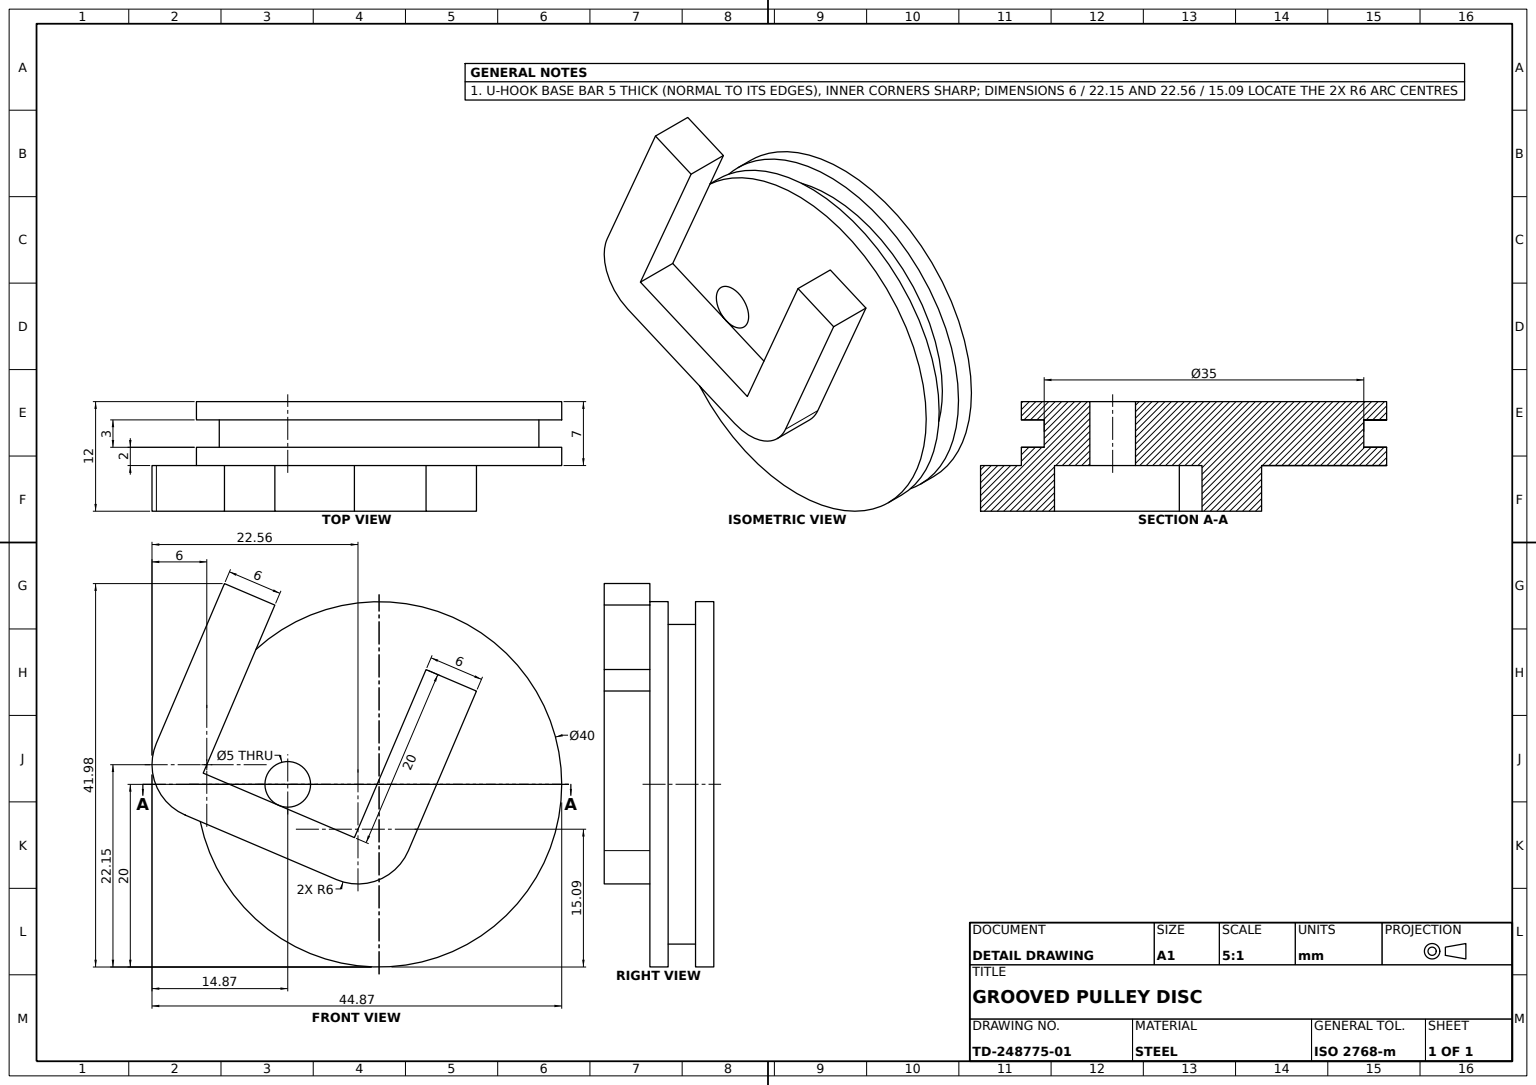
from build123d import *

# Parameters (mm, degrees)
DISC_PROFILE_40_R      = 20
DISC_40X7_DEPTH        = 3.5
RIM_GROOVE_PROFILE_W   = 3
RIM_GROOVE_PROFILE_H   = 2.5
THROUGH_HOLE_PROFILE_R = 2.5
THROUGH_HOLE_DEPTH     = 47
U_HOOK_BOSS_DEPTH      = 5


with BuildPart() as part:
    # Disc Profile Ø40 → Disc Ø40x7 (new, symmetric)
    with BuildSketch(Plane.XY):
        Circle(DISC_PROFILE_40_R)
    extrude(amount=DISC_40X7_DEPTH, both=True)

    # Rim Groove Profile → Rim Groove (revolve, cut)
    with BuildSketch(Plane(origin=(0, 0, 0), x_dir=(0, 0, -1), z_dir=(1, 0, 0)), mode=Mode.PRIVATE) as rim_groove_sk:
        with Locations((0, 18.75)):
            Rectangle(RIM_GROOVE_PROFILE_W, RIM_GROOVE_PROFILE_H)
    revolve(rim_groove_sk.sketch.rotate(Axis((0, 0, 14.756637323), (0, 0, -1)), 90), axis=Axis((0, 0, 14.756637323), (0, 0, -1)), mode=Mode.SUBTRACT)

    # Through Hole Profile → Through Hole (cut)
    with BuildSketch(Plane.XY.offset(3.5)):
        with Locations((-10, 0)):
            Circle(THROUGH_HOLE_PROFILE_R)
    extrude(amount=-THROUGH_HOLE_DEPTH, mode=Mode.SUBTRACT)

    # U Hook Profile → U Hook Boss (add)
    with BuildSketch(Plane.XY.offset(3.5)):
        with BuildLine():
            Line((-19.259231956, 1.231512725), (-2.70246973, -5.830613343))
            Line((-2.70246973, -5.830613343), (5.144337012, 12.56578913))
            Line((5.144337012, 12.56578913), (10.663257754, 10.211747107))
            Line((10.663257754, 10.211747107), (3.208791349, -7.264835242))
            ThreePointArc((3.208791349, -7.264835242), (-0.072222189, -10.477818578), (-4.664171415, -10.429713961))
            Line((-4.664171415, -10.429713961), (-21.220933641, -3.367587893))
            ThreePointArc((-21.220933641, -3.367587893), (-24.433916977, -0.086574356), (-24.38581236, 4.505374871))
            Line((-24.38581236, 4.505374871), (-16.931345956, 21.981957221))
            Line((-16.931345956, 21.981957221), (-11.412425214, 19.627915198))
            Line((-11.412425214, 19.627915198), (-19.259231956, 1.231512725))
        make_face()
    extrude(amount=U_HOOK_BOSS_DEPTH)


solid = part.part
